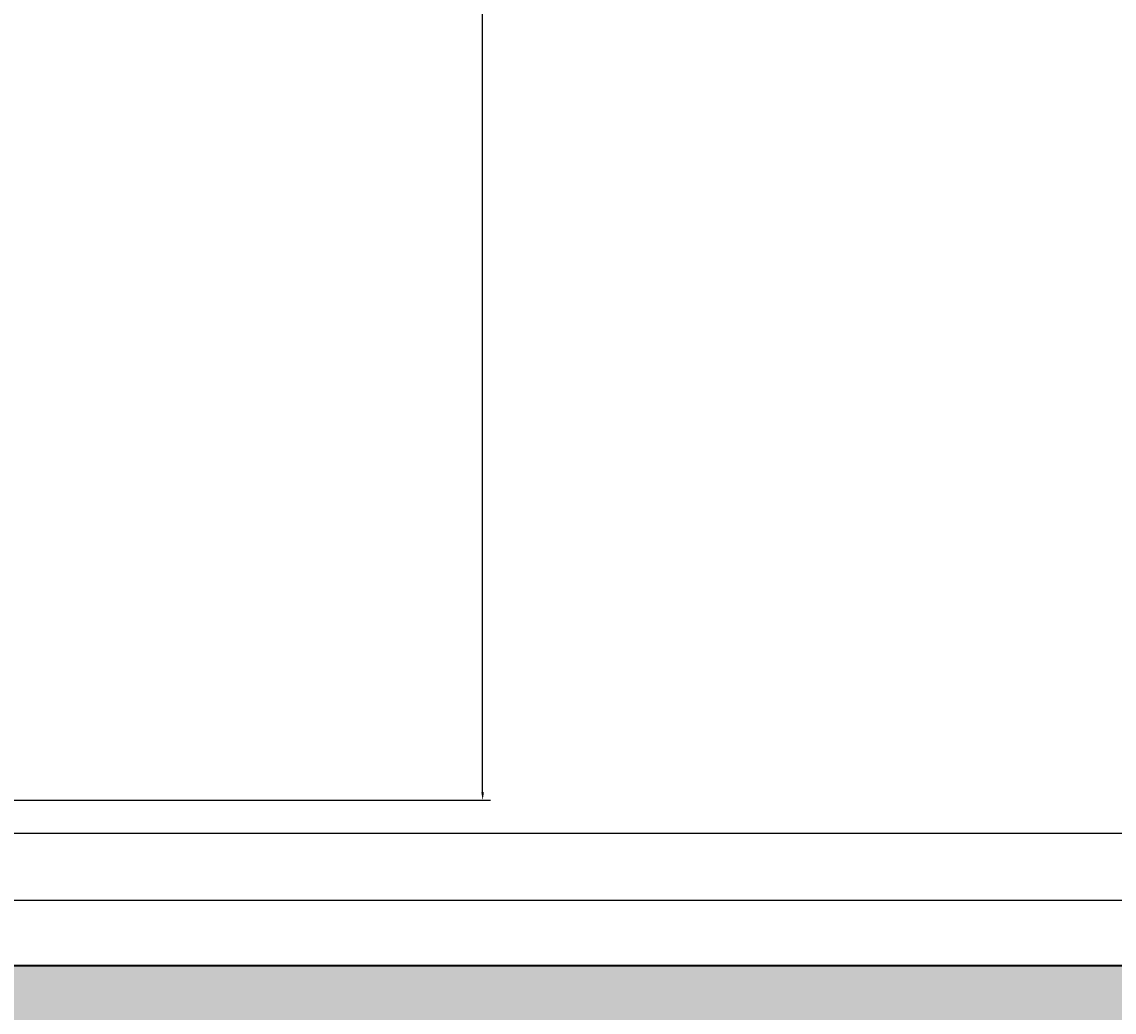
# Model space of a CAD drawing. Units: inches. Extents: x 1998 to 2588, y 1139 to 1977.
# Tile 45 of 134: x 2257 to 2282, y 1592 to 1615. Entities that reach past the tile are written whole.
import ezdxf

# ---------------------------------------------------------------- set-up
doc = ezdxf.new("R2010")
doc.units = ezdxf.units.IN
for name, color, linetype, lineweight in [('A-ANNO-DIMS', 2, 'Continuous', 18), ('A-WALL-PATT', 252, 'Continuous', 13), ('WALL', 200, 'Continuous', 35)]:
    doc.layers.add(name, color=color, linetype=linetype, lineweight=lineweight)
doc.styles.get("Standard").update_dxf_attribs({"font": 'arial.ttf'})
doc.dimstyles.get("Standard").update_dxf_attribs({"dimtxt": 0.18, "dimasz": 0.18, "dimexe": 0.18, "dimexo": 0.0625, "dimgap": 0.09, "dimtad": 0, "dimtih": 1, "dimtoh": 1, "dimdec": 4, "dimzin": 0, "dimdsep": 46, "dimtxsty": 'Standard', "dimcen": 0.09, "dimadec": 0, "dimazin": 0, "dimtfac": 1, "dimtdec": 4, "dimtofl": 0, "dimtmove": 0, "dimatfit": 3, "dimfxl": 1, "dimtolj": 1, "dimtzin": 0, "dimarcsym": 0})

# ---------------------------------------------------------------- blocks, each defined once
blk = doc.blocks.new('*D11')
at = {"layer": 'A-ANNO-DIMS', "color": 0, "lineweight": -2, "transparency": 16777216}
for p, q in [((2256.378, 1671.356), (2267.646, 1671.356)), ((2267.466, 1671.176), (2267.466, 1634.372)), ((2267.466, 1597.201), (2267.466, 1634.005)), ((2256.378, 1597.021), (2267.646, 1597.021))]:
    blk.add_line(p, q, dxfattribs=at)
at = {"layer": 'A-ANNO-DIMS', "color": 0, "transparency": 16777216}
for points in [[(2267.436, 1671.176), (2267.496, 1671.176), (2267.466, 1671.356)], [(2267.436, 1597.201), (2267.496, 1597.201), (2267.466, 1597.021)]]:
    blk.add_solid(points, dxfattribs=at)
at = {"layer": 'Defpoints', "color": 0, "transparency": 16777216}
for p in [(2256.316, 1671.356), (2256.316, 1597.021), (2267.466, 1597.021)]:
    blk.add_point(p, dxfattribs=at)
at = {"layer": 'A-ANNO-DIMS', "color": 0, "transparency": 16777216, "insert": (2267.466, 1634.189), "char_height": 0.18, "attachment_point": 5}
blk.add_mtext('\\A1;SOFA 74 TYP.', dxfattribs=at)
blk = doc.blocks.new('*D30')
at = {"layer": 'A-ANNO-DIMS', "color": 0, "lineweight": -2, "transparency": 16777216}
for p, q in [((2407.91, 1636.732), (1997.843, 1636.732)), ((1998.023, 1636.552), (1998.023, 1615.913)), ((1998.023, 1594.912), (1998.023, 1615.552)), ((2407.91, 1594.732), (1997.843, 1594.732))]:
    blk.add_line(p, q, dxfattribs=at)
at = {"layer": 'A-ANNO-DIMS', "color": 0, "transparency": 16777216}
for points in [[(1997.993, 1636.552), (1998.053, 1636.552), (1998.023, 1636.732)], [(1997.993, 1594.912), (1998.053, 1594.912), (1998.023, 1594.732)]]:
    blk.add_solid(points, dxfattribs=at)
at = {"layer": 'Defpoints', "color": 0, "transparency": 16777216}
for p in [(1998.023, 1636.732), (2407.973, 1636.732), (2407.973, 1594.732)]:
    blk.add_point(p, dxfattribs=at)
at = {"layer": 'A-ANNO-DIMS', "color": 0, "transparency": 16777216, "insert": (1998.023, 1615.732), "char_height": 0.18, "attachment_point": 5}
blk.add_mtext('\\A1;42', dxfattribs=at)
blk = doc.blocks.new('*D34')
at = {"layer": 'A-ANNO-DIMS', "color": 0, "lineweight": -2, "transparency": 16777216}
for p, q in [((2407.91, 1594.732), (1997.843, 1594.732)), ((1998.023, 1594.552), (1998.023, 1558.913)), ((1998.023, 1522.912), (1998.023, 1558.552)), ((2407.91, 1522.732), (1997.843, 1522.732))]:
    blk.add_line(p, q, dxfattribs=at)
at = {"layer": 'A-ANNO-DIMS', "color": 0, "transparency": 16777216}
for points in [[(1997.993, 1594.552), (1998.053, 1594.552), (1998.023, 1594.732)], [(1997.993, 1522.912), (1998.053, 1522.912), (1998.023, 1522.732)]]:
    blk.add_solid(points, dxfattribs=at)
at = {"layer": 'Defpoints', "color": 0, "transparency": 16777216}
for p in [(1998.023, 1594.732), (2407.973, 1594.732), (2407.973, 1522.732)]:
    blk.add_point(p, dxfattribs=at)
at = {"layer": 'A-ANNO-DIMS', "color": 0, "transparency": 16777216, "insert": (1998.023, 1558.732), "char_height": 0.18, "attachment_point": 5}
blk.add_mtext('\\A1;72', dxfattribs=at)
blk = doc.blocks.new('*D39')
at = {"layer": 'A-ANNO-DIMS', "color": 0, "lineweight": -2, "transparency": 16777216}
for p, q in [((2115.035, 1628.742), (2588.309, 1628.742)), ((2588.129, 1628.562), (2588.129, 1612.685)), ((2588.129, 1596.444), (2588.129, 1612.321)), ((2115.035, 1596.264), (2588.309, 1596.264))]:
    blk.add_line(p, q, dxfattribs=at)
at = {"layer": 'A-ANNO-DIMS', "color": 0, "transparency": 16777216}
for points in [[(2588.099, 1628.562), (2588.159, 1628.562), (2588.129, 1628.742)], [(2588.099, 1596.444), (2588.159, 1596.444), (2588.129, 1596.264)]]:
    blk.add_solid(points, dxfattribs=at)
at = {"layer": 'Defpoints', "color": 0, "transparency": 16777216}
for p in [(2114.973, 1628.742), (2588.129, 1628.742), (2114.973, 1596.264)]:
    blk.add_point(p, dxfattribs=at)
at = {"layer": 'A-ANNO-DIMS', "color": 0, "transparency": 16777216, "insert": (2588.129, 1612.503), "char_height": 0.18, "attachment_point": 5}
blk.add_mtext('\\A1;32.48', dxfattribs=at)

msp = doc.modelspace()

# ---------------------------------------------------------------- hatches: boundary and pattern name
at = {"layer": 'A-WALL-PATT'}
h = msp.add_hatch(color=256, dxfattribs=at)
h.dxf.hatch_style = 1
h.paths.add_polyline_path([(2222.9729, 1888.7324), (2099.4125, 1888.7324), (2099.4125, 1879.7324), (2222.9729, 1879.7324)])
h.paths.add_polyline_path([(2096.9729, 1868.3278), (2087.9729, 1868.3278), (2087.9729, 1775.637), (2096.9729, 1775.637)])
h.paths.add_polyline_path([(2227.4729, 1868.3278), (2222.9729, 1868.3278), (2222.9729, 1774.3318), (2227.4729, 1774.3318)])
h.paths.add_polyline_path([(2188.3019, 1759.7324), (2138.6074, 1759.7324), (2099.4125, 1759.7324), (2099.4125, 1755.2324), (2176.9729, 1755.2324), (2188.3019, 1755.2324)])
h.paths.add_polyline_path([(2087.9729, 1759.7324), (2059.4729, 1759.7324), (2059.4729, 1702.7324), (2087.9729, 1702.7324), (2087.9729, 1707.2324), (2063.9729, 1707.2324), (2063.9729, 1755.2324), (2087.9729, 1755.2324)])
h.paths.add_polyline_path([(2096.9729, 1755.2324), (2087.9729, 1755.2324), (2087.9729, 1707.2324), (2096.9729, 1707.2324)])
h.paths.add_polyline_path([(2187.0461, 1707.2324), (2105.9729, 1707.2324), (2096.9729, 1707.2324), (2087.9729, 1707.2324), (2087.9729, 1702.7324), (2105.9729, 1702.7324), (2114.9729, 1702.7324), (2187.0461, 1702.7324)])
h.paths.add_polyline_path([(2181.4729, 1719.2028), (2176.9729, 1719.2028), (2176.9729, 1707.2324), (2181.4729, 1707.2324)])
h.paths.add_polyline_path([(2216.0332, 1588.7324), (2114.9729, 1588.7324), (2105.9729, 1588.7324), (2105.9729, 1584.2324), (2216.0332, 1584.2324)])
h.paths.add_polyline_path([(2077.691, 1588.7324), (2061.4729, 1588.7324), (2061.4729, 1584.2324), (2077.691, 1584.2324)])
h.paths.add_polyline_path([(2105.9729, 1588.7324), (2098.0956, 1588.7324), (2098.0956, 1584.2324), (2105.9729, 1584.2324)])
h.paths.add_polyline_path([(2114.9729, 1596.2642), (2110.1012, 1596.2642), (2105.9729, 1596.2642), (2105.9729, 1588.7324), (2114.9729, 1588.7324)])
h.paths.add_polyline_path([(2114.9729, 1584.2324), (2105.9729, 1584.2324), (2105.9729, 1580.249), (2110.1012, 1580.249), (2114.9729, 1580.249)])
h.paths.add_polyline_path([(2114.9729, 1547.7716), (2110.1012, 1547.7716, -0.0318759), (2105.9729, 1548.035), (2105.9729, 1470.2324), (2108.3775, 1470.2324), (2108.3775, 1465.7324), (2186.2943, 1465.7324), (2186.2943, 1470.2324), (2114.9729, 1470.2324)])
h.paths.add_polyline_path([(2227.4729, 1584.2324), (2222.9729, 1584.2324), (2222.9729, 1486.137), (2227.4729, 1486.137)])
h.paths.add_polyline_path([(2295.4138, 1593.2324), (2227.4729, 1593.2324), (2227.4729, 1588.7324), (2295.4138, 1588.7324), (2295.4138, 1591.8729)])
h.paths.add_polyline_path([(2345.9729, 1627.1165), (2341.4729, 1627.1165), (2341.4729, 1593.2324), (2337.2869, 1593.2324), (2337.2869, 1591.8729), (2337.2869, 1588.7324), (2345.9729, 1588.7324)])
h.paths.add_polyline_path([(2291.9729, 1588.7324), (2287.4729, 1588.7324), (2287.4729, 1522.7324), (2291.9729, 1522.7324)])
h.paths.add_polyline_path([(2291.9729, 1522.7324), (2287.4729, 1522.7324), (2227.4729, 1522.7324), (2227.4729, 1518.2324), (2291.9729, 1518.2324)])
h.paths.add_polyline_path([(2295.7347, 1519.5919), (2295.7347, 1522.7324), (2291.9729, 1522.7324), (2291.9729, 1518.2324), (2295.7347, 1518.2324)])
h.paths.add_polyline_path([(2345.9729, 1522.7324), (2337.6078, 1522.7324), (2337.6078, 1519.5919), (2337.6078, 1518.2324), (2341.4729, 1518.2324), (2341.4729, 1488.5616), (2345.9729, 1488.5616)])
h.paths.add_polyline_path([(2345.9729, 1468.1569), (2341.4729, 1468.1569), (2341.4729, 1374.2324), (2227.4729, 1374.2324), (2227.4729, 1369.7324), (2345.9729, 1369.7324)])
h.paths.add_polyline_path([(2345.9729, 1369.7324), (2341.4729, 1369.7324), (2341.4729, 1362.2324), (2345.9729, 1362.2324)])
h.paths.add_polyline_path([(2345.9729, 1317.7324), (2345.9729, 1322.2324), (2341.4729, 1322.2324), (2341.4729, 1285.137), (2345.9729, 1285.137)], flags=17)
h.paths.add_polyline_path([(2356.2096, 1322.2324), (2345.9729, 1322.2324), (2345.9729, 1317.7324), (2356.2096, 1317.7324), (2356.2096, 1319.3088)], flags=17)
h.paths.add_polyline_path([(2393.9729, 1322.2324), (2375.6999, 1322.2324), (2375.6999, 1319.3088, -0.0202458), (2375.636, 1317.7324), (2393.9729, 1317.7324)], flags=17)
h.paths.add_polyline_path([(2398.4729, 1322.2324), (2393.9729, 1322.2324), (2393.9729, 1317.7324), (2393.9729, 1237.7324), (2345.9729, 1237.7324), (2345.9729, 1264.7324), (2341.4729, 1264.7324), (2341.4729, 1228.7324), (2393.9729, 1228.7324), (2482.7412, 1228.7324), (2482.7412, 1237.7324), (2398.4729, 1237.7324), (2398.4729, 1297.1029)])
h.paths.add_polyline_path([(2398.4729, 1362.2324), (2393.9729, 1362.2324), (2393.9729, 1357.7324), (2398.4729, 1357.7324)])
h.paths.add_polyline_path([(2345.9729, 1329.7549), (2341.4729, 1329.7549), (2341.4729, 1322.2324), (2345.9729, 1322.2324)])

# ---------------------------------------------------------------- linework, layer by layer
at = {"layer": 'WALL'}
msp.add_line((2296.3298, 1593.2324), (2227.4729, 1593.2324), dxfattribs=at)

# ---------------------------------------------------------------- dimensions: what is measured, and where the dimension line sits
at = {"layer": 'A-ANNO-DIMS'}
dim = msp.add_linear_dim(base=(2267.4662, 1597.0205), p1=(2256.3158, 1671.3565), p2=(2256.3158, 1597.0205), angle=270, text='SOFA <> TYP.', dimstyle='Standard', override={"dimdec": 0, "dimlfac": 1, "dimrnd": 0, "dimzin": 0, "dimdsep": 46, "dimlunit": 2}, dxfattribs=at)
dim.commit()
dim.dimension.update_dxf_attribs({"geometry": '*D11', "text_midpoint": (2267.4662, 1634.1885)})
for base, p1, p2, override, picture, middle in [((1998.0229, 1636.7324), (2407.9729, 1594.7324), (2407.9729, 1636.7324), {"dimdec": 0, "dimlfac": 1, "dimrnd": 0, "dimzin": 0, "dimdsep": 46, "dimlunit": 2}, '*D30', (1998.0229, 1615.7324)), ((2588.1286, 1628.7416), (2114.9729, 1596.2642), (2114.9729, 1628.7416), {"dimdec": 2, "dimlfac": 1, "dimrnd": 0, "dimzin": 0, "dimdsep": 46, "dimlunit": 2}, '*D39', (2588.1286, 1612.5029)), ((1998.0229, 1594.7324), (2407.9729, 1522.7324), (2407.9729, 1594.7324), {"dimdec": 0, "dimlfac": 1, "dimrnd": 0, "dimzin": 0, "dimdsep": 46, "dimlunit": 2}, '*D34', (1998.0229, 1558.7324))]:
    dim = msp.add_linear_dim(base=base, p1=p1, p2=p2, angle=90, dimstyle='Standard', override=override, dxfattribs=at)
    dim.commit()
    dim.dimension.update_dxf_attribs({"geometry": picture, "text_midpoint": middle})

doc.saveas('drawing.dxf')
